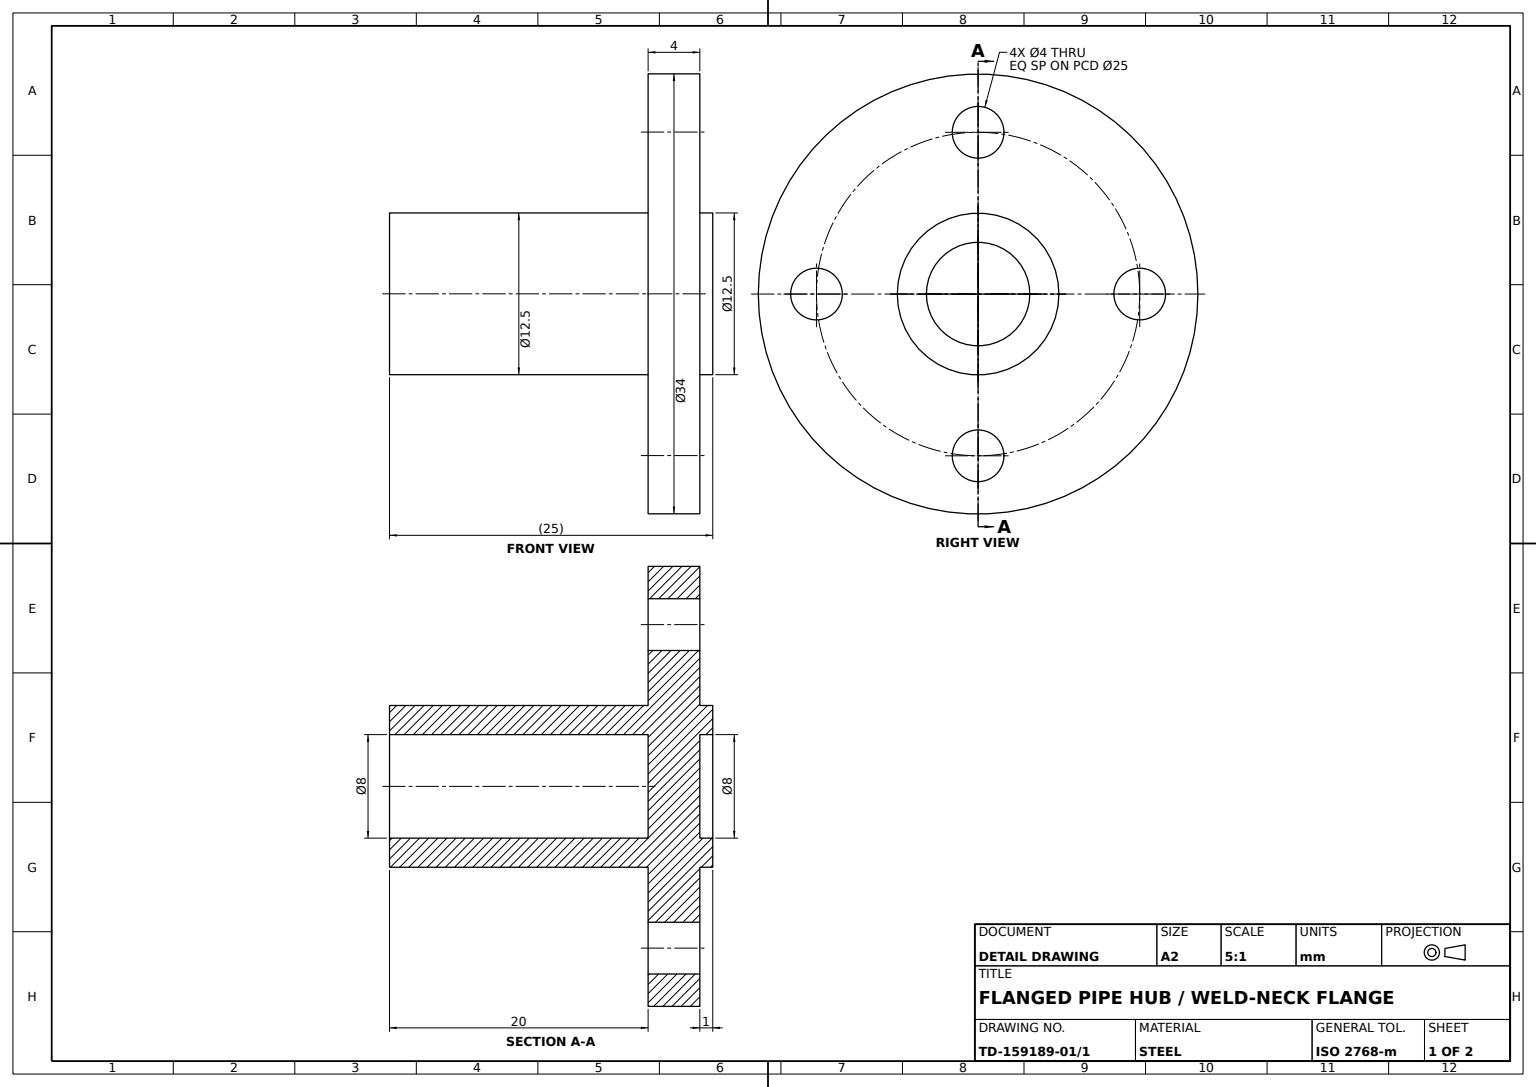
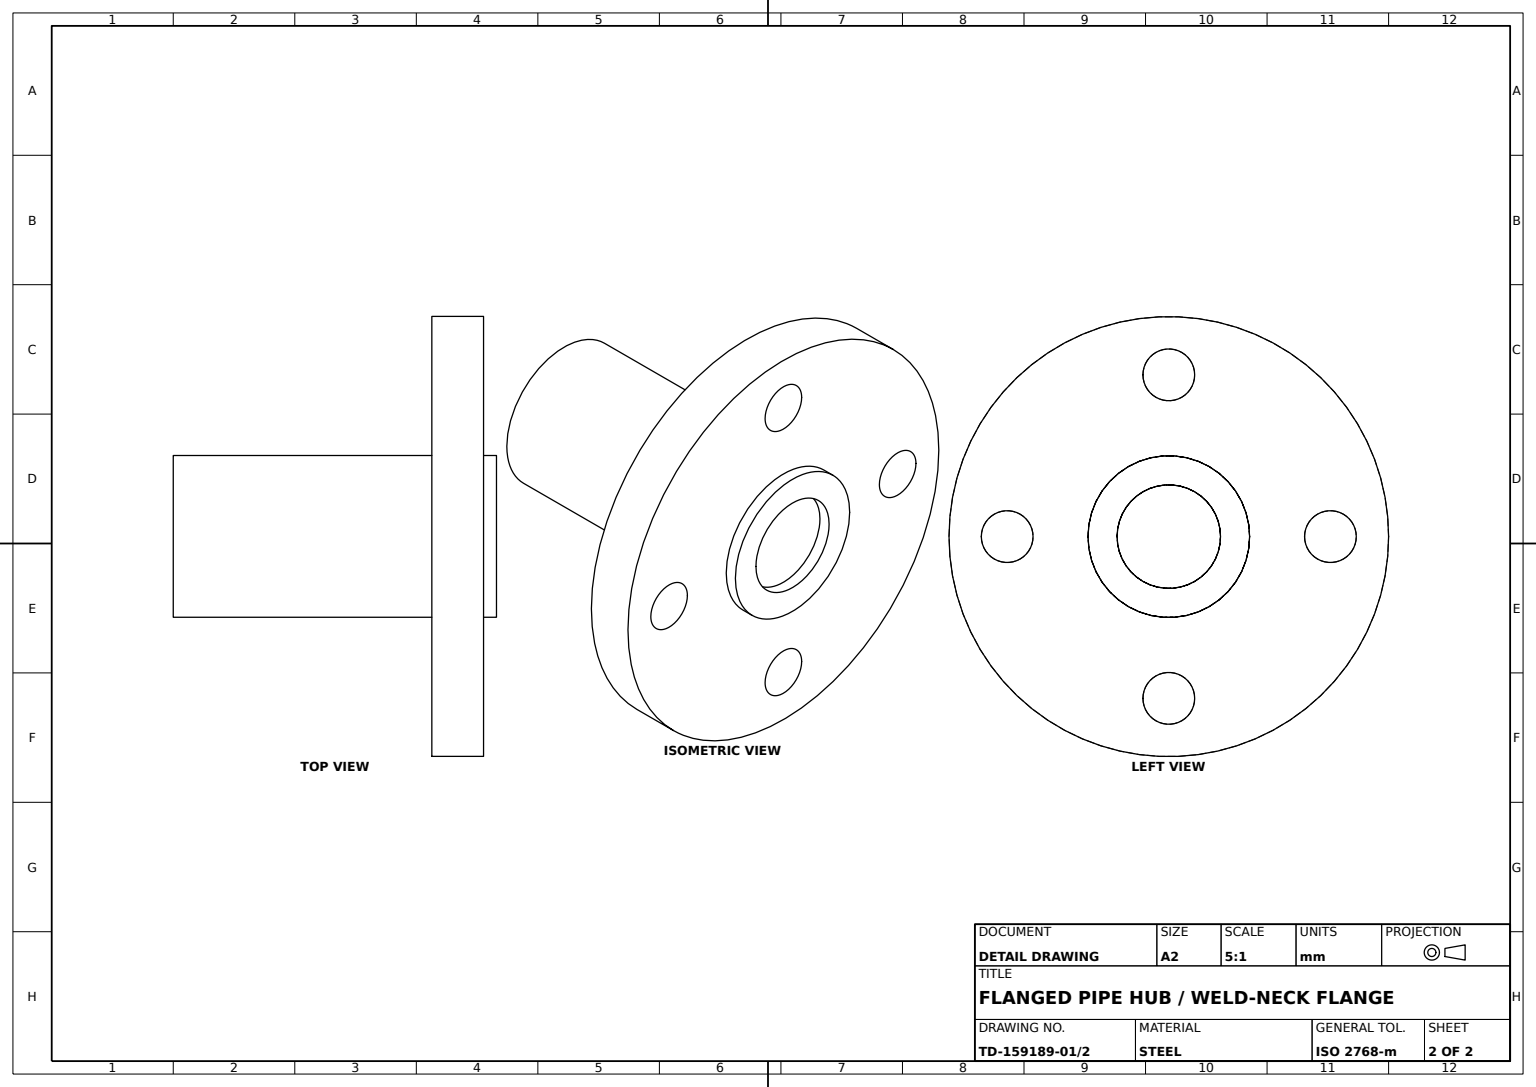
from build123d import *

# Parameters (mm, degrees)
FLANGE_PROFILE_SKETCH_R = 17
FLANGE_34X4_DEPTH       = 4
HUB_PROFILE_SKETCH_R    = 6.25
HUB_PROFILE_SKETCH_R_2  = 4
HUB_TUBE_20MM_DEPTH     = 20
BOLT_HOLES_SKETCH_R     = 2
BOLT_HOLES_4X_DEPTH     = 4
REAR_START              = 1
REAR_SPIGOT_SKETCH_R    = 6.25
REAR_SPIGOT_SKETCH_R_2  = 4
REAR_SPIGOT_1MM_DEPTH   = 1


with BuildPart() as part:
    # Flange Profile Sketch → Flange Ø34x4 (new body)
    with BuildSketch(Plane.XY):
        Circle(FLANGE_PROFILE_SKETCH_R)
    extrude(amount=FLANGE_34X4_DEPTH)

    # Hub Profile Sketch → Hub Tube 20mm (add)
    with BuildSketch(Plane.XY.offset(4)):
        Circle(HUB_PROFILE_SKETCH_R)
        Circle(HUB_PROFILE_SKETCH_R_2, mode=Mode.SUBTRACT)
    extrude(amount=HUB_TUBE_20MM_DEPTH)

    # Bolt Holes Sketch → Bolt Holes 4x (cut)
    with BuildSketch(Plane.XY.offset(4)):
        with Locations((0, 12.5)):
            Circle(BOLT_HOLES_SKETCH_R)
        with Locations((12.5, 0)):
            Circle(BOLT_HOLES_SKETCH_R)
        with Locations((0, -12.5)):
            Circle(BOLT_HOLES_SKETCH_R)
        with Locations((-12.5, 0)):
            Circle(BOLT_HOLES_SKETCH_R)
    extrude(amount=-BOLT_HOLES_4X_DEPTH, mode=Mode.SUBTRACT)

    # Rear Spigot Sketch → Rear Spigot 1mm (add)
    with BuildSketch(Plane(origin=(0, 0, 0), x_dir=(-1, 0, 0), z_dir=(0, 0, -1)).offset(REAR_START)):
        with Locations(Location((0, 0, 0), (0, 0, 180))):
            Circle(REAR_SPIGOT_SKETCH_R)
        with Locations(Location((0, 0, 0), (0, 0, 180))):
            Circle(REAR_SPIGOT_SKETCH_R_2, mode=Mode.SUBTRACT)
    extrude(amount=-REAR_SPIGOT_1MM_DEPTH)


solid = part.part
